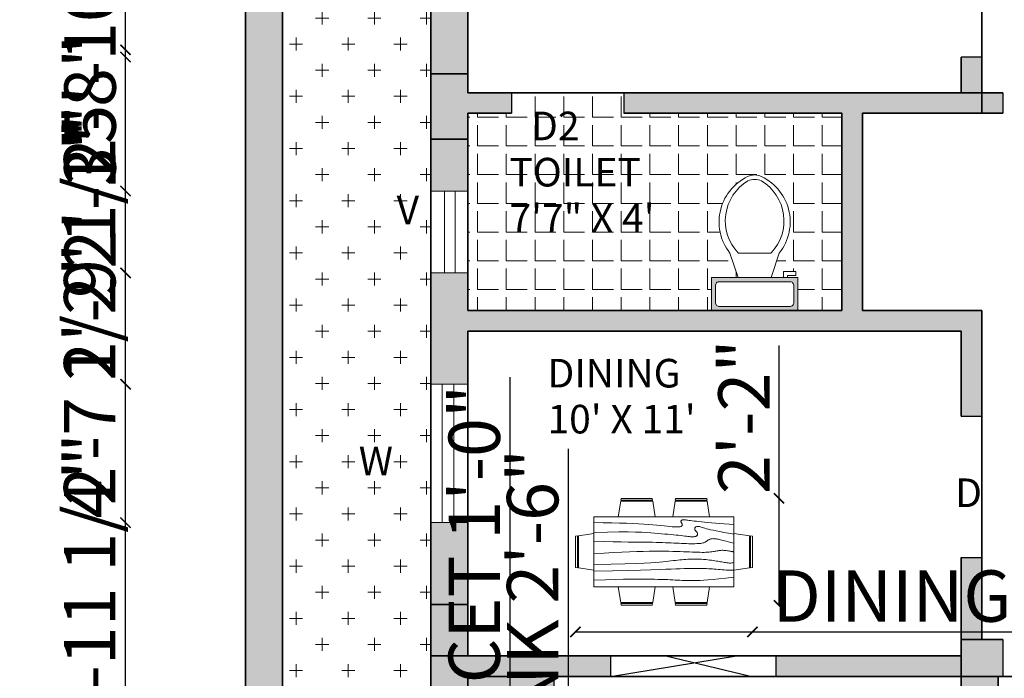
# Model space of a CAD drawing. Units: inches. Extents: x 1858 to 2399, y 1317 to 1943.
# Tile 2 of 8: x 1858 to 2098, y 1554 to 1714. Entities that reach past the tile are written whole.
import ezdxf

# ---------------------------------------------------------------- set-up
doc = ezdxf.new("R2010")
doc.units = ezdxf.units.IN
for name, color, linetype, lineweight in [('A-ANNO-DIMS', 2, 'Continuous', 18), ('A-ANNO-TEXT', 7, 'Continuous', 18), ('A-AREA-IDEN', 7, 'Continuous', 18), ('A-COLS', 7, 'Continuous', 35), ('A-COLS-PATT', 5, 'Continuous', 13), ('A-DOOR', 4, 'Continuous', 25), ('A-FLOR-CASE', 8, 'Continuous', 25), ('A-FLOR-FIXT', 9, 'Continuous', 18), ('A-FLOR-FIXT-PATT', 9, 'Continuous', 13), ('A-FLOR-PATT', 8, 'Continuous', 13), ('A-FURN', 8, 'Continuous', 18), ('A-WALL', 7, 'Continuous', 35), ('A-WALL-PATT', 1, 'Continuous', 13), ('L-SITE-PATT', 8, 'Continuous', 13), ('window', 4, 'Continuous', 18)]:
    doc.layers.add(name, color=color, linetype=linetype, lineweight=lineweight)
doc.styles.get("Standard").update_dxf_attribs({"font": 'arial.ttf'})
doc.dimstyles.new('ISO-25', dxfattribs={"dimtxt": 12.5, "dimasz": 2.5, "dimexe": 1.25, "dimexo": 0.625, "dimtad": 1, "dimdec": 0, "dimlunit": 4, "dimtxsty": 'Standard', "dimblk": 'ARCHTICK', "dimcen": 2.5, "dimse1": 1, "dimse2": 1, "dimclrd": 3, "dimclrt": 4, "dimadec": 0, "dimazin": 0, "dimtfac": 1, "dimtdec": 0, "dimtmove": 0, "dimatfit": 3, "dimfxl": 1, "dimarcsym": 0})

# ---------------------------------------------------------------- blocks, each defined once
blk = doc.blocks.new('*U4')
for p, q in [((9.5, -6), (9.5, -2)), ((-10, -8.5), (-8, -8.5)), ((-10, -9.5), (-10, -8.5)), ((-7, -9.5), (-10, -9.5)), ((-8, -8.5), (-8, -8)), ((-7, -8), (-7, -9.5)), ((-4, -8), (-6, -14)), ((4, -8), (6, -14)), ((4, -14), (-4, -14))]:
    blk.add_line(p, q)
blk.add_lwpolyline([(10.5, -8), (10.5, 0), (-10.5, 0), (-10.5, -8)], close=True)
for points in [[(-9.5, -2), (-9.5, -6)], [(8.5, -1), (-8.5, -1)], [(-8.5, -7), (8.5, -7)]]:
    blk.add_lwpolyline(points)
for centre, radius, start, end in [((-8.62, -1.88), 0.884, 81.8699, 188.1301), ((8.62, -1.88), 0.884, 351.8699, 98.1301), ((-8.62, -6.12), 0.884, 171.8699, 278.1301), ((8.62, -6.12), 0.884, 261.8699, 8.1301), ((3.52, -21.58), 12.17, 141.4691, 247.9714), ((4.2, -21.82), 11.33, 136.3677, 238.9468), ((-3.52, -21.58), 12.17, 292.0284, 38.5307), ((-4.2, -21.82), 11.33, 301.053, 43.6321), ((0, -27.88), 4, 245.7318, 294.2682), ((0, -29), 4, 254.8605, 285.1395)]:
    blk.add_arc(centre, radius, start, end)
blk = doc.blocks.new('Dining Set - 36 x 72 in.')
for p, q in [((-22.2343, 26.00059), (-23.4847, 17.99762)), ((-22.2304, 26), (-5.7608, 26)), ((-22, 27.5), (-22.1562, 26.50042)), ((-5.8416, 26.5), (-22.1534, 26.5)), ((-22, 27.5), (-6, 27.5)), ((-5.8437, 26.49966), (-6, 27.5)), ((-4.5152, 17.99762), (-5.7655, 25.99926)), ((5.7657, 26.00059), (4.5153, 17.99762)), ((5.7696, 26), (22.2392, 26)), ((6, 27.5), (5.8438, 26.50042)), ((22.1584, 26.5), (5.8466, 26.5)), ((6, 27.5), (22, 27.5)), ((22.1563, 26.49966), (22, 27.5)), ((23.4848, 17.99762), (22.2345, 25.99926)), ((36, 18), (-36, 18)), ((-36, 18), (-36, -18)), ((36, -18), (36, 18)), ((-45.5, 8), (-44.5004, 8.15617)), ((-45.5, 8), (-45.5, -8)), ((-44.5, -8.15843), (-44.5, 8.15338)), ((-44.0006, 8.23428), (-35.9976, 9.48474)), ((-44, 8.23041), (-44, -8.23915)), ((44.0006, 8.23428), (35.9976, 9.48474)), ((44, 8.23041), (44, -8.23915)), ((44.5, -8.15843), (44.5, 8.15338)), ((45.5, 8), (44.5005, 8.15617)), ((45.5, 8), (45.5, -8)), ((-44.4997, -8.15631), (-45.5, -8)), ((-35.9976, -9.48476), (-43.9993, -8.2345)), ((35.9976, -9.48476), (43.9993, -8.2345)), ((44.4997, -8.15631), (45.5, -8)), ((-36, -18), (36, -18)), ((-22.2343, -26.0006), (-23.4847, -17.99762)), ((-4.5152, -17.99762), (-5.7655, -25.99928)), ((5.7657, -26.0006), (4.5153, -17.99762)), ((23.4848, -17.99762), (22.2345, -25.99928)), ((-22.2304, -26), (-5.7608, -26)), ((-22, -27.5), (-22.1562, -26.50044)), ((-5.8416, -26.5), (-22.1534, -26.5)), ((-22, -27.5), (-6, -27.5)), ((-5.8437, -26.49967), (-6, -27.5)), ((5.7696, -26), (22.2392, -26)), ((6, -27.5), (5.8438, -26.50044)), ((22.1584, -26.5), (5.8466, -26.5)), ((6, -27.5), (22, -27.5)), ((22.1563, -26.49967), (22, -27.5))]:
    blk.add_line(p, q)
for points in [[(-36, 15), (-31.1772, 14.97754), (-26.8079, 14.91406), (-22.8538, 14.81543), (-19.276, 14.6875), (-16.0362, 14.53613), (-13.0957, 14.36718), (-10.4159, 14.18652), (-7.9583, 14), (-5.6904, 13.81315), (-3.6035, 13.63021), (-1.6954, 13.45508), (0.0365, 13.29166), (1.5945, 13.14388), (2.9811, 13.01562), (4.1988, 12.9108), (5.25, 12.83333), (6.1393, 12.78613), (6.8802, 12.76823), (7.4883, 12.77767), (7.9792, 12.8125), (8.3685, 12.87077), (8.6719, 12.95052), (8.9049, 13.0498), (9.0833, 13.16666), (9.2205, 13.29899), (9.3216, 13.44401), (9.3895, 13.59879), (9.4271, 13.76041), (9.4373, 13.92594), (9.4232, 14.09245), (9.3875, 14.257), (9.3333, 14.41666), (9.2638, 14.56917), (9.1836, 14.71484), (9.0975, 14.85465), (9.0104, 14.98958), (8.9272, 15.1206), (8.8529, 15.2487), (8.7922, 15.37483), (8.75, 15.5), (8.7305, 15.62467), (8.7344, 15.74739), (8.7617, 15.86621), (8.8125, 15.97916), (8.8867, 16.08431), (8.9844, 16.17968), (9.1055, 16.26334), (9.25, 16.33333), (9.4189, 16.38802), (9.6172, 16.42708), (9.8506, 16.45052), (10.125, 16.45833), (10.4463, 16.45052), (10.8203, 16.42708), (11.2529, 16.38802), (11.75, 16.33333), (12.3184, 16.26318), (12.9694, 16.17838), (13.7151, 16.07991), (14.5677, 15.96875), (15.5395, 15.84586), (16.6426, 15.71224), (17.8893, 15.56884), (19.2917, 15.41666), (20.859, 15.25667), (22.5879, 15.08984), (24.4721, 14.91715), (26.5052, 14.73958), (28.6809, 14.5581), (30.9929, 14.3737), (33.4347, 14.18733), (36, 14)], [(-36, 10), (-28.9766, 10.14274), (-23.1725, 10.20442), (-18.4241, 10.19775), (-14.5677, 10.13541), (-11.4399, 10.03011), (-8.877, 9.89453), (-6.7154, 9.74137), (-4.7917, 9.58333), (-2.9698, 9.43082), (-1.2246, 9.28515), (0.4415, 9.14534), (2.026, 9.01041), (3.5266, 8.87939), (4.9408, 8.7513), (6.266, 8.62516), (7.5, 8.5), (8.6411, 8.37549), (9.6914, 8.2539), (10.6538, 8.13818), (11.5312, 8.03125), (12.3267, 7.93603), (13.043, 7.85547), (13.6831, 7.79248), (14.25, 7.75), (14.7471, 7.7303), (15.1797, 7.73307), (15.5537, 7.75732), (15.875, 7.80208), (16.1494, 7.86637), (16.3828, 7.94922), (16.5811, 8.04964), (16.75, 8.16666), (16.8944, 8.29915), (17.0143, 8.44531), (17.1089, 8.60319), (17.1771, 8.77083), (17.218, 8.94629), (17.2305, 9.1276), (17.2137, 9.31282), (17.1667, 9.5), (17.0895, 9.6875), (16.987, 9.875), (16.8649, 10.0625), (16.7292, 10.25), (16.5856, 10.4375), (16.4401, 10.625), (16.2985, 10.8125), (16.1667, 11), (16.05, 11.18733), (15.9518, 11.3737), (15.8752, 11.5581), (15.8229, 11.73958), (15.798, 11.91715), (15.8034, 12.08984), (15.842, 12.25667), (15.9167, 12.41666), (16.0295, 12.56836), (16.1784, 12.70833), (16.3605, 12.83268), (16.5729, 12.9375), (16.8127, 13.01888), (17.0768, 13.07291), (17.3625, 13.0957), (17.6667, 13.08333), (17.9894, 13.03312), (18.3418, 12.94726), (18.7382, 12.82918), (19.1927, 12.68229), (19.7195, 12.51001), (20.3327, 12.31575), (21.0465, 12.10294), (21.875, 11.875), (22.8357, 11.63354), (23.959, 11.37304), (25.2786, 11.08618), (26.8282, 10.76562), (28.6414, 10.40405), (30.752, 9.99414), (33.1936, 9.52856), (36, 9)], [(-36, 5.5), (-30.7157, 5.3348), (-26.069, 5.20963), (-21.9946, 5.11767), (-18.4271, 5.05208), (-15.3009, 5.00602), (-12.5508, 4.97265), (-10.1112, 4.94515), (-7.9167, 4.91666), (-5.909, 4.88167), (-4.0586, 4.83984), (-2.3429, 4.79215), (-0.7396, 4.73958), (0.7739, 4.6831), (2.22, 4.6237), (3.6213, 4.56233), (5, 4.5), (6.373, 4.43782), (7.7344, 4.3776), (9.0723, 4.32129), (10.375, 4.27083), (11.6309, 4.22819), (12.8281, 4.19531), (13.9551, 4.17415), (15, 4.16666), (15.954, 4.17448), (16.819, 4.19791), (17.6001, 4.23698), (18.3021, 4.29166), (18.9299, 4.36198), (19.4883, 4.44791), (19.9823, 4.54948), (20.4167, 4.66666), (20.7969, 4.79899), (21.1302, 4.94401), (21.4245, 5.09879), (21.6875, 5.26041), (21.9271, 5.42594), (22.1511, 5.59245), (22.3672, 5.757), (22.5834, 5.91666), (22.8065, 6.06868), (23.0404, 6.21093), (23.2879, 6.34147), (23.5521, 6.45833), (23.8358, 6.55957), (24.142, 6.64323), (24.4735, 6.70735), (24.8334, 6.75), (25.2235, 6.76969), (25.642, 6.76692), (26.0858, 6.74267), (26.5521, 6.69791), (27.0379, 6.63362), (27.5404, 6.55078), (28.0565, 6.45036), (28.5834, 6.33333), (29.1242, 6.19987), (29.7071, 6.04687), (30.3661, 5.87044), (31.1354, 5.66666), (32.0493, 5.43164), (33.142, 5.16146), (34.4475, 4.85221), (36, 4.5)], [(-36, -1), (-30.7915, -0.6591), (-26.0195, -0.38216), (-21.6519, -0.16284), (-17.6563, 0.00521), (-14.0005, 0.12833), (-10.6523, 0.21289), (-7.5796, 0.26522), (-4.75, 0.29166), (-2.134, 0.29793), (0.2878, 0.28711), (2.5317, 0.26163), (4.6146, 0.22396), (6.5529, 0.17651), (8.3633, 0.12174), (10.0623, 0.06209), (11.6667, 0), (13.1899, -0.06201), (14.6341, -0.1211), (15.9982, -0.17432), (17.2813, -0.21875), (18.4823, -0.25147), (19.6003, -0.26953), (20.6343, -0.27002), (21.5834, -0.25), (22.4481, -0.20768), (23.2357, -0.14584), (23.9549, -0.06836), (24.6146, 0.02083), (25.2235, 0.11784), (25.7904, 0.21875), (26.3241, 0.31966), (26.8334, 0.41666), (27.3265, 0.50618), (27.8099, 0.58593), (28.2894, 0.65397), (28.7709, 0.70833), (29.2601, 0.74707), (29.763, 0.76823), (30.2855, 0.76985), (30.8334, 0.75), (31.4088, 0.70784), (31.9994, 0.64713), (32.589, 0.57275), (33.1615, 0.48958), (33.7008, 0.4025), (34.1908, 0.3164), (34.6153, 0.23616), (34.9584, 0.16666), (35.2099, 0.11165), (35.3848, 0.07031), (35.504, 0.04069), (35.5886, 0.02083), (35.6594, 0.00879), (35.7377, 0.0026), (35.8442, 0.00032), (36, 0)], [(-36, -6.5), (-27.1843, -6.31267), (-20.084, -6.1263), (-14.469, -5.9419), (-10.1094, -5.76042), (-6.7752, -5.58285), (-4.2363, -5.41016), (-2.2629, -5.24333), (-0.625, -5.08334), (0.8708, -4.93099), (2.2715, -4.78646), (3.5872, -4.64974), (4.8281, -4.52084), (6.0046, -4.39974), (7.127, -4.28646), (8.2053, -4.18099), (9.25, -4.08334), (10.2705, -3.99382), (11.2734, -3.91407), (12.2647, -3.84603), (13.25, -3.79167), (14.2354, -3.75293), (15.2266, -3.73177), (16.2295, -3.73015), (17.25, -3.75), (18.2912, -3.79248), (19.3451, -3.85547), (20.4009, -3.93604), (21.4479, -4.03125), (22.4754, -4.13819), (23.4727, -4.25391), (24.4289, -4.37549), (25.3334, -4.5), (26.1785, -4.62492), (26.9694, -4.74935), (27.7145, -4.87281), (28.4219, -4.99479), (29.1, -5.11483), (29.7572, -5.23242), (30.4016, -5.34709), (31.0417, -5.45834), (31.6837, -5.56437), (32.3262, -5.65821), (32.9658, -5.73153), (33.599, -5.77604), (34.2224, -5.78345), (34.8327, -5.74545), (35.4264, -5.65373), (36, -5.5)], [(-36, -10), (-26.4022, -9.81299), (-18.4675, -9.62891), (-11.9839, -9.45069), (-6.7396, -9.28125), (-2.5226, -9.12354), (0.8789, -8.98047), (3.6769, -8.85498), (6.0833, -8.75), (8.2767, -8.66765), (10.3021, -8.60677), (12.1712, -8.56543), (13.8958, -8.54167), (15.4876, -8.53353), (16.9583, -8.53907), (18.3197, -8.55632), (19.5834, -8.58334), (20.7616, -8.61841), (21.8685, -8.66081), (22.9188, -8.71004), (23.9271, -8.76563), (24.9081, -8.82707), (25.8763, -8.89388), (26.8465, -8.96558), (27.8334, -9.04167), (28.8474, -9.12118), (29.8828, -9.20117), (30.93, -9.27824), (31.9792, -9.34896), (33.0205, -9.40991), (34.0443, -9.45768), (35.0407, -9.48885), (36, -9.5)], [(-36, -14.5), (-30.0881, -14.33513), (-25.0332, -14.21224), (-20.7312, -14.12647), (-17.0781, -14.07292), (-13.97, -14.04671), (-11.3027, -14.04297), (-8.9724, -14.05681), (-6.875, -14.08334), (-4.9224, -14.11833), (-3.0905, -14.16016), (-1.3709, -14.20785), (0.2448, -14.26042), (1.7647, -14.3169), (3.1973, -14.3763), (4.5507, -14.43767), (5.8333, -14.5), (7.0554, -14.5621), (8.235, -14.62175), (9.3922, -14.67652), (10.5469, -14.72396), (11.7192, -14.76164), (12.929, -14.78711), (14.1965, -14.79794), (15.5417, -14.79167), (16.9933, -14.76424), (18.6152, -14.70508), (20.4804, -14.60197), (22.6615, -14.44271), (25.2312, -14.21509), (28.2624, -13.9069), (31.8277, -13.50594), (36, -13)]]:
    blk.add_lwpolyline(points)
blk = doc.blocks.new('_ArchTick')
at = {"color": 0, "linetype": 'ByBlock', "const_width": 0.15}
blk.add_lwpolyline([(-0.5, -0.5), (0.5, 0.5)], dxfattribs=at)
blk = doc.blocks.new('*D21')
at = {"layer": 'A-ANNO-DIMS', "color": 3, "lineweight": -2, "transparency": 16777216}
for p, q in [((1991.88, 1527.2), (1991.88, 1609.72)), ((1991.88, 1497.2), (1991.88, 1527.2))]:
    blk.add_line(p, q, dxfattribs=at)
at = {"layer": 'Defpoints', "color": 0, "transparency": 16777216}
for p in [(1987.38, 1527.2), (1991.88, 1527.2), (1987.38, 1497.2)]:
    blk.add_point(p, dxfattribs=at)
at = {"layer": 'A-ANNO-DIMS', "color": 3, "lineweight": -2, "transparency": 16777216, "xscale": 2.5, "yscale": 2.5, "zscale": 2.5}
for p, rotation in [((1991.88, 1527.2), 90), ((1991.88, 1497.2), 270)]:
    blk.add_blockref('_ArchTick', p, dxfattribs=dict(at, rotation=rotation))
at = {"layer": 'A-ANNO-DIMS', "color": 4, "transparency": 16777216, "insert": (1984.79, 1569.71), "char_height": 12.5, "attachment_point": 5, "rotation": 90}
blk.add_mtext('SINK 2\'-6"', dxfattribs=at)
blk = doc.blocks.new('*D23')
at = {"layer": 'A-ANNO-DIMS', "color": 3, "lineweight": -2, "transparency": 16777216}
for p, q in [((1977.68, 1516.18), (1977.68, 1627.15)), ((1977.68, 1504.18), (1977.68, 1516.18))]:
    blk.add_line(p, q, dxfattribs=at)
at = {"layer": 'Defpoints', "color": 0, "transparency": 16777216}
for p in [(1975.88, 1516.18), (1977.68, 1516.18), (1975.88, 1504.18)]:
    blk.add_point(p, dxfattribs=at)
at = {"layer": 'A-ANNO-DIMS', "color": 3, "lineweight": -2, "transparency": 16777216, "xscale": 2.5, "yscale": 2.5, "zscale": 2.5}
for p, rotation in [((1977.68, 1516.18), 90), ((1977.68, 1504.18), 270)]:
    blk.add_blockref('_ArchTick', p, dxfattribs=dict(at, rotation=rotation))
at = {"layer": 'A-ANNO-DIMS', "color": 4, "transparency": 16777216, "insert": (1970.59, 1572.91), "char_height": 12.5, "attachment_point": 5, "rotation": 90}
blk.add_mtext('FAUCET 1\'-0"', dxfattribs=at)
blk = doc.blocks.new('*D25')
at = {"layer": 'A-ANNO-DIMS', "color": 3, "lineweight": -2, "transparency": 16777216}
for p, q in [((1993.57, 1565.17), (2036.62, 1565.17)), ((2036.62, 1565.17), (2177.76, 1565.17))]:
    blk.add_line(p, q, dxfattribs=at)
at = {"layer": 'Defpoints', "color": 0, "transparency": 16777216}
for p in [(1993.57, 1571.63), (2036.62, 1571.63), (2036.62, 1565.17)]:
    blk.add_point(p, dxfattribs=at)
at = {"layer": 'A-ANNO-DIMS', "color": 3, "lineweight": -2, "transparency": 16777216, "xscale": 2.5, "yscale": 2.5, "zscale": 2.5, "rotation": 180}
blk.add_blockref('_ArchTick', (1993.57, 1565.17), dxfattribs=at)
at = {"layer": 'A-ANNO-DIMS', "color": 3, "lineweight": -2, "transparency": 16777216, "xscale": 2.5, "yscale": 2.5, "zscale": 2.5}
blk.add_blockref('_ArchTick', (2036.62, 1565.17), dxfattribs=at)
at = {"layer": 'A-ANNO-DIMS', "color": 4, "transparency": 16777216, "insert": (2108.44, 1572.26), "char_height": 12.5, "attachment_point": 5}
blk.add_mtext('DINING SET 3\'-7"', dxfattribs=at)
blk = doc.blocks.new('*D26')
at = {"layer": 'A-ANNO-DIMS', "color": 3, "lineweight": -2, "transparency": 16777216}
for p, q in [((2043.08, 1597.65), (2043.08, 1634.84)), ((2043.08, 1571.63), (2043.08, 1597.65))]:
    blk.add_line(p, q, dxfattribs=at)
at = {"layer": 'Defpoints', "color": 0, "transparency": 16777216}
for p in [(2036.62, 1597.65), (2043.08, 1597.65), (2036.62, 1571.63)]:
    blk.add_point(p, dxfattribs=at)
at = {"layer": 'A-ANNO-DIMS', "color": 3, "lineweight": -2, "transparency": 16777216, "xscale": 2.5, "yscale": 2.5, "zscale": 2.5}
for p, rotation in [((2043.08, 1597.65), 90), ((2043.08, 1571.63), 270)]:
    blk.add_blockref('_ArchTick', p, dxfattribs=dict(at, rotation=rotation))
at = {"layer": 'A-ANNO-DIMS', "color": 4, "transparency": 16777216, "insert": (2036.18, 1617.49), "char_height": 12.5, "attachment_point": 5, "rotation": 90}
blk.add_mtext('2\'-2"', dxfattribs=at)
blk = doc.blocks.new('*D31')
at = {"layer": 'A-ANNO-DIMS', "color": 3, "lineweight": -2, "transparency": 16777216}
for p, q in [((1967.38, 1917.54), (1988.35, 1917.54)), ((1988.35, 1917.54), (2024.15, 1917.54))]:
    blk.add_line(p, q, dxfattribs=at)
at = {"layer": 'Defpoints', "color": 0, "transparency": 16777216}
for p in [(1988.35, 1917.54), (1967.38, 1554.34), (1988.35, 1554.34)]:
    blk.add_point(p, dxfattribs=at)
at = {"layer": 'A-ANNO-DIMS', "color": 3, "lineweight": -2, "transparency": 16777216, "xscale": 2.5, "yscale": 2.5, "zscale": 2.5, "rotation": 180}
blk.add_blockref('_ArchTick', (1967.38, 1917.54), dxfattribs=at)
at = {"layer": 'A-ANNO-DIMS', "color": 3, "lineweight": -2, "transparency": 16777216, "xscale": 2.5, "yscale": 2.5, "zscale": 2.5}
blk.add_blockref('_ArchTick', (1988.35, 1917.54), dxfattribs=at)
at = {"layer": 'A-ANNO-DIMS', "color": 4, "transparency": 16777216, "insert": (2007.5, 1924.55), "char_height": 12.5, "attachment_point": 5}
blk.add_mtext('1\'-9"', dxfattribs=at)
blk = doc.blocks.new('*D40')
at = {"layer": 'A-ANNO-DIMS', "color": 3, "lineweight": -2, "transparency": 16777216}
for p, q in [((1884.18, 1536.07), (1884.18, 1611.87)), ((1884.18, 1488.33), (1884.18, 1536.07))]:
    blk.add_line(p, q, dxfattribs=at)
at = {"layer": 'Defpoints', "color": 0, "transparency": 16777216}
for p in [(1884.18, 1536.07), (1958.38, 1536.07), (1958.38, 1488.33)]:
    blk.add_point(p, dxfattribs=at)
at = {"layer": 'A-ANNO-DIMS', "color": 3, "lineweight": -2, "transparency": 16777216, "xscale": 2.5, "yscale": 2.5, "zscale": 2.5}
for p, rotation in [((1884.18, 1536.07), 90), ((1884.18, 1488.33), 270)]:
    blk.add_blockref('_ArchTick', p, dxfattribs=dict(at, rotation=rotation))
at = {"layer": 'A-ANNO-DIMS', "color": 4, "transparency": 16777216, "insert": (1877.08, 1575.22), "char_height": 12.5, "attachment_point": 5, "rotation": 90}
blk.add_mtext('3\'-11 1/2"', dxfattribs=at)
blk = doc.blocks.new('*D41')
at = {"layer": 'A-ANNO-DIMS', "color": 3, "lineweight": -2, "transparency": 16777216}
for p, q in [((1884.18, 1591.74), (1884.18, 1658.34)), ((1884.18, 1536.07), (1884.18, 1591.74))]:
    blk.add_line(p, q, dxfattribs=at)
at = {"layer": 'Defpoints', "color": 0, "transparency": 16777216}
for p in [(1884.18, 1591.74), (1958.38, 1591.74), (1958.38, 1536.07)]:
    blk.add_point(p, dxfattribs=at)
at = {"layer": 'A-ANNO-DIMS', "color": 3, "lineweight": -2, "transparency": 16777216, "xscale": 2.5, "yscale": 2.5, "zscale": 2.5}
for p, rotation in [((1884.18, 1591.74), 90), ((1884.18, 1536.07), 270)]:
    blk.add_blockref('_ArchTick', p, dxfattribs=dict(at, rotation=rotation))
at = {"layer": 'A-ANNO-DIMS', "color": 4, "transparency": 16777216, "insert": (1877.09, 1626.29), "char_height": 12.5, "attachment_point": 5, "rotation": 90}
blk.add_mtext('4\'-7 1/2"', dxfattribs=at)
blk = doc.blocks.new('*D42')
at = {"layer": 'A-ANNO-DIMS', "color": 3, "lineweight": -2, "transparency": 16777216}
for p, q in [((1884.18, 1625.4), (1884.18, 1691.71)), ((1884.18, 1591.74), (1884.18, 1625.4))]:
    blk.add_line(p, q, dxfattribs=at)
at = {"layer": 'Defpoints', "color": 0, "transparency": 16777216}
for p in [(1884.18, 1625.4), (1958.38, 1625.4), (1958.38, 1591.74)]:
    blk.add_point(p, dxfattribs=at)
at = {"layer": 'A-ANNO-DIMS', "color": 3, "lineweight": -2, "transparency": 16777216, "xscale": 2.5, "yscale": 2.5, "zscale": 2.5}
for p, rotation in [((1884.18, 1625.4), 90), ((1884.18, 1591.74), 270)]:
    blk.add_blockref('_ArchTick', p, dxfattribs=dict(at, rotation=rotation))
at = {"layer": 'A-ANNO-DIMS', "color": 4, "transparency": 16777216, "insert": (1877.09, 1659.8), "char_height": 12.5, "attachment_point": 5, "rotation": 90}
blk.add_mtext('2\'-9 1/2"', dxfattribs=at)
blk = doc.blocks.new('*D43')
at = {"layer": 'A-ANNO-DIMS', "color": 3, "lineweight": -2, "transparency": 16777216}
for p, q in [((1884.18, 1652.51), (1884.18, 1689.7)), ((1884.18, 1625.4), (1884.18, 1652.51))]:
    blk.add_line(p, q, dxfattribs=at)
at = {"layer": 'Defpoints', "color": 0, "transparency": 16777216}
for p in [(1884.18, 1652.51), (1958.38, 1652.51), (1958.38, 1625.4)]:
    blk.add_point(p, dxfattribs=at)
at = {"layer": 'A-ANNO-DIMS', "color": 3, "lineweight": -2, "transparency": 16777216, "xscale": 2.5, "yscale": 2.5, "zscale": 2.5}
for p, rotation in [((1884.18, 1652.51), 90), ((1884.18, 1625.4), 270)]:
    blk.add_blockref('_ArchTick', p, dxfattribs=dict(at, rotation=rotation))
at = {"layer": 'A-ANNO-DIMS', "color": 4, "transparency": 16777216, "insert": (1877.16, 1672.36), "char_height": 12.5, "attachment_point": 5, "rotation": 90}
blk.add_mtext('2\'-3"', dxfattribs=at)
blk = doc.blocks.new('*D44')
at = {"layer": 'A-ANNO-DIMS', "color": 3, "lineweight": -2, "transparency": 16777216}
for p, q in [((1884.18, 1672.42), (1884.18, 1708.22)), ((1884.18, 1652.51), (1884.18, 1672.42))]:
    blk.add_line(p, q, dxfattribs=at)
at = {"layer": 'Defpoints', "color": 0, "transparency": 16777216}
for p in [(1884.18, 1672.42), (1958.38, 1672.42), (1958.38, 1652.51)]:
    blk.add_point(p, dxfattribs=at)
at = {"layer": 'A-ANNO-DIMS', "color": 3, "lineweight": -2, "transparency": 16777216, "xscale": 2.5, "yscale": 2.5, "zscale": 2.5}
for p, rotation in [((1884.18, 1672.42), 90), ((1884.18, 1652.51), 270)]:
    blk.add_blockref('_ArchTick', p, dxfattribs=dict(at, rotation=rotation))
at = {"layer": 'A-ANNO-DIMS', "color": 4, "transparency": 16777216, "insert": (1877.17, 1691.57), "char_height": 12.5, "attachment_point": 5, "rotation": 90}
blk.add_mtext('1\'-8"', dxfattribs=at)
blk = doc.blocks.new('*D45')
at = {"layer": 'A-ANNO-DIMS', "color": 3, "lineweight": -2, "transparency": 16777216}
blk.add_line((1884.18, 1672.42), (1884.18, 1742.58), dxfattribs=at)
at = {"layer": 'Defpoints', "color": 0, "transparency": 16777216}
for p in [(1884.18, 1742.58), (1958.38, 1742.58), (1958.38, 1672.42)]:
    blk.add_point(p, dxfattribs=at)
at = {"layer": 'A-ANNO-DIMS', "color": 3, "lineweight": -2, "transparency": 16777216, "xscale": 2.5, "yscale": 2.5, "zscale": 2.5}
for p, rotation in [((1884.18, 1742.58), 90), ((1884.18, 1672.42), 270)]:
    blk.add_blockref('_ArchTick', p, dxfattribs=dict(at, rotation=rotation))
at = {"layer": 'A-ANNO-DIMS', "color": 4, "transparency": 16777216, "insert": (1877.17, 1707.5), "char_height": 12.5, "attachment_point": 5, "rotation": 90}
blk.add_mtext('5\'-10"', dxfattribs=at)
blk = doc.blocks.new('*D50')
at = {"layer": 'A-ANNO-DIMS', "color": 3, "lineweight": -2, "transparency": 16777216}
for p, q in [((2097.46, 1917.54), (2127.41, 1917.54)), ((2127.41, 1917.54), (2164.6, 1917.54))]:
    blk.add_line(p, q, dxfattribs=at)
at = {"layer": 'Defpoints', "color": 0, "transparency": 16777216}
for p in [(2127.41, 1917.54), (2097.46, 1563.34), (2127.41, 1563.34)]:
    blk.add_point(p, dxfattribs=at)
at = {"layer": 'A-ANNO-DIMS', "color": 3, "lineweight": -2, "transparency": 16777216, "xscale": 2.5, "yscale": 2.5, "zscale": 2.5, "rotation": 180}
blk.add_blockref('_ArchTick', (2097.46, 1917.54), dxfattribs=at)
at = {"layer": 'A-ANNO-DIMS', "color": 3, "lineweight": -2, "transparency": 16777216, "xscale": 2.5, "yscale": 2.5, "zscale": 2.5}
blk.add_blockref('_ArchTick', (2127.41, 1917.54), dxfattribs=at)
at = {"layer": 'A-ANNO-DIMS', "color": 4, "transparency": 16777216, "insert": (2147.25, 1924.55), "char_height": 12.5, "attachment_point": 5}
blk.add_mtext('2\'-6"', dxfattribs=at)
blk = doc.blocks.new('*D56')
at = {"layer": 'A-ANNO-DIMS', "color": 3, "lineweight": -2, "transparency": 16777216}
for p, q in [((1977.99, 1917.54), (2005.38, 1917.54)), ((2005.38, 1917.54), (2071.7, 1917.54))]:
    blk.add_line(p, q, dxfattribs=at)
at = {"layer": 'Defpoints', "color": 0, "transparency": 16777216}
for p in [(2005.38, 1917.54), (1977.99, 1696.34), (2005.38, 1696.34)]:
    blk.add_point(p, dxfattribs=at)
at = {"layer": 'A-ANNO-DIMS', "color": 3, "lineweight": -2, "transparency": 16777216, "xscale": 2.5, "yscale": 2.5, "zscale": 2.5, "rotation": 180}
blk.add_blockref('_ArchTick', (1977.99, 1917.54), dxfattribs=at)
at = {"layer": 'A-ANNO-DIMS', "color": 3, "lineweight": -2, "transparency": 16777216, "xscale": 2.5, "yscale": 2.5, "zscale": 2.5}
blk.add_blockref('_ArchTick', (2005.38, 1917.54), dxfattribs=at)
at = {"layer": 'A-ANNO-DIMS', "color": 4, "transparency": 16777216, "insert": (2039.79, 1924.63), "char_height": 12.5, "attachment_point": 5}
blk.add_mtext('2\'-3 1/2"', dxfattribs=at)
blk = doc.blocks.new('*D57')
at = {"layer": 'A-ANNO-DIMS', "color": 3, "lineweight": -2, "transparency": 16777216}
for p, q in [((1884.18, 1729.93), (1884.18, 1767.12)), ((1884.18, 1705.02), (1884.18, 1729.93))]:
    blk.add_line(p, q, dxfattribs=at)
at = {"layer": 'Defpoints', "color": 0, "transparency": 16777216}
for p in [(1884.18, 1729.93), (2087.38, 1729.93), (2087.38, 1705.02)]:
    blk.add_point(p, dxfattribs=at)
at = {"layer": 'A-ANNO-DIMS', "color": 3, "lineweight": -2, "transparency": 16777216, "xscale": 2.5, "yscale": 2.5, "zscale": 2.5}
for p, rotation in [((1884.18, 1729.93), 90), ((1884.18, 1705.02), 270)]:
    blk.add_blockref('_ArchTick', p, dxfattribs=dict(at, rotation=rotation))
at = {"layer": 'A-ANNO-DIMS', "color": 4, "transparency": 16777216, "insert": (1877.28, 1749.77), "char_height": 12.5, "attachment_point": 5, "rotation": 90}
blk.add_mtext('2\'-1"', dxfattribs=at)
blk = doc.blocks.new('*D58')
at = {"layer": 'A-ANNO-DIMS', "color": 3, "lineweight": -2, "transparency": 16777216}
for p, q in [((1884.18, 1730.57), (1884.18, 1767.76)), ((1884.18, 1706.78), (1884.18, 1730.57))]:
    blk.add_line(p, q, dxfattribs=at)
at = {"layer": 'Defpoints', "color": 0, "transparency": 16777216}
for p in [(1884.18, 1730.57), (2145.38, 1730.57), (2145.38, 1706.78)]:
    blk.add_point(p, dxfattribs=at)
at = {"layer": 'A-ANNO-DIMS', "color": 3, "lineweight": -2, "transparency": 16777216, "xscale": 2.5, "yscale": 2.5, "zscale": 2.5}
for p, rotation in [((1884.18, 1730.57), 90), ((1884.18, 1706.78), 270)]:
    blk.add_blockref('_ArchTick', p, dxfattribs=dict(at, rotation=rotation))
at = {"layer": 'A-ANNO-DIMS', "color": 4, "transparency": 16777216, "insert": (1877.17, 1750.41), "char_height": 12.5, "attachment_point": 5, "rotation": 90}
blk.add_mtext('2\'-0"', dxfattribs=at)
blk = doc.blocks.new('*D59')
at = {"layer": 'A-ANNO-DIMS', "color": 3, "lineweight": -2, "transparency": 16777216}
for p, q in [((2302.58, 1617.63), (2302.58, 1693.66)), ((2302.58, 1583.24), (2302.58, 1617.63))]:
    blk.add_line(p, q, dxfattribs=at)
at = {"layer": 'Defpoints', "color": 0, "transparency": 16777216}
for p in [(2092.38, 1617.63), (2302.58, 1617.63), (2092.38, 1583.24)]:
    blk.add_point(p, dxfattribs=at)
at = {"layer": 'A-ANNO-DIMS', "color": 3, "lineweight": -2, "transparency": 16777216, "xscale": 2.5, "yscale": 2.5, "zscale": 2.5}
for p, rotation in [((2302.58, 1617.63), 90), ((2302.58, 1583.24), 270)]:
    blk.add_blockref('_ArchTick', p, dxfattribs=dict(at, rotation=rotation))
at = {"layer": 'A-ANNO-DIMS', "color": 4, "transparency": 16777216, "insert": (2295.49, 1656.89), "char_height": 12.5, "attachment_point": 5, "rotation": 90}
blk.add_mtext('2\'-10 1/2"', dxfattribs=at)

msp = doc.modelspace()

# ---------------------------------------------------------------- hatches: boundary and pattern name
at = {"layer": 'A-COLS-PATT'}
h = msp.add_hatch(color=256, dxfattribs=at)
h.dxf.hatch_style = 1
h.paths.add_polyline_path([(1977.99, 1696.34), (1967.38, 1696.34), (1967.38, 1700.89), (1958.38, 1700.89), (1958.38, 1685.05), (1967.38, 1685.05), (1967.38, 1691.34), (1977.99, 1691.34)])
h.paths.add_polyline_path([(1967.38, 1571.83), (1958.38, 1571.83), (1958.38, 1559.34), (1967.38, 1559.34)])
h.paths.add_polyline_path([(1977.97, 1476.34), (1967.38, 1476.34), (1967.38, 1482.01), (1958.38, 1474.25), (1958.38, 1467.34), (1967.38, 1467.34)])
h.paths.add_polyline_path([(2096.38, 1473.96), (2087.38, 1481.51), (2087.38, 1476.34), (2084.48, 1476.34), (2089.85, 1467.34), (2096.38, 1467.34)])
h.paths.add_polyline_path([(2273.38, 1837.34), (2265.79, 1837.34), (2258.24, 1828.34), (2264.38, 1828.34), (2264.38, 1823.36), (2273.38, 1827.14)])
h.paths.add_polyline_path([(2097.64, 1837.34), (2082.58, 1837.34), (2082.58, 1828.34), (2097.64, 1828.34)])
h.paths.add_polyline_path([(1977.66, 1837.34), (1949.42, 1837.34), (1949.42, 1828.34), (1977.66, 1828.34)])
h = msp.add_hatch(color=256, dxfattribs=at)
h.dxf.hatch_style = 1
h.paths.add_polyline_path([(2092.38, 1705.02), (2087.38, 1705.02), (2087.38, 1696.34), (2092.38, 1696.34)])
h.paths.add_polyline_path([(2097.51, 1696.34), (2092.38, 1696.34), (2092.38, 1691.34), (2097.51, 1691.34)])
h.paths.add_polyline_path([(2140.38, 1696.34), (2135.36, 1696.34), (2135.36, 1691.34), (2140.38, 1691.34)])
h.paths.add_polyline_path([(2145.38, 1706.78), (2140.38, 1706.78), (2140.38, 1696.34), (2145.38, 1696.34)])
h.paths.add_polyline_path([(2097.46, 1563.34), (2092.38, 1563.34), (2087.38, 1563.34), (2087.38, 1554.34), (2096.38, 1554.34), (2097.46, 1554.34)])
at = {"layer": 'A-FLOR-FIXT-PATT'}
h = msp.add_hatch(color=256, dxfattribs=at)
h.dxf.hatch_style = 1
h.set_gradient(color1=(0, 0, 255), color2=(255, 255, 0))
h.paths.add_polyline_path([(2010.03, 1501.34), (2040.03, 1501.34), (2040.03, 1477.34), (2034.03, 1477.34), (2034.03, 1476.34), (2038.03, 1476.34), (2050.44, 1476.34), (2056.5, 1476.34), (2056.5, 1507.28), (1988.35, 1507.28), (1988.35, 1554.34), (1967.38, 1554.34), (1967.38, 1525.7, -0.414214), (1968.88, 1527.2), (1985.88, 1527.2, -0.414214), (1987.38, 1525.7), (1987.38, 1498.7, -0.414214), (1985.88, 1497.2), (1968.88, 1497.2, -0.414214), (1967.38, 1498.7), (1967.38, 1476.34), (2016.03, 1476.34), (2016.03, 1477.34), (2010.03, 1477.34)])
h.paths.add_polyline_path([(2129, 1826.59, 0.414214), (2128, 1827.34), (2110.75, 1827.34, 0.414214), (2110, 1826.34), (2110, 1822.09, 0.414214), (2111, 1821.34), (2128.25, 1821.34, 0.414214), (2129, 1822.34)])
h.paths.add_polyline_path([(2047.65, 1651.34), (2026.65, 1651.34), (2026.65, 1643.34), (2047.65, 1643.34)])
h.paths.add_polyline_path([(2045.65, 1644.34, 0.5), (2046.65, 1645.34), (2046.65, 1649.34, 0.5), (2045.65, 1650.34), (2028.65, 1650.34, 0.5), (2027.65, 1649.34), (2027.65, 1645.34, 0.5), (2028.65, 1644.34)], flags=16)
at = {"layer": 'A-FLOR-PATT'}
h = msp.add_hatch(dxfattribs=at)
h.set_pattern_fill('ANGLE', color=256)
h.set_pattern_definition([(0, (0, 0), (0, 6.985), [5.08, -1.905]), (90, (0, 0), (-6.985, 4e-16), [5.08, -1.905])])
h.paths.add_polyline_path([(2058.38, 1691.34), (2005.38, 1691.34), (2005.38, 1696.34), (1977.99, 1696.34), (1977.99, 1691.34), (1967.38, 1691.34), (1967.38, 1643.34), (2026.65, 1643.34), (2026.65, 1651.34), (2033.15, 1651.34), (2031.15, 1657.34, -0.501323), (2036.1, 1676.2, -0.132891), (2038.19, 1676.2, -0.501317), (2043.15, 1657.34), (2041.15, 1651.34), (2044.15, 1651.34), (2044.15, 1652.84), (2047.15, 1652.84), (2047.15, 1651.34), (2047.65, 1651.34), (2047.65, 1643.34), (2058.38, 1643.34)])
h.paths.add_polyline_path([(2140.38, 1828.34), (2130, 1828.34), (2130, 1820.34), (2123.5, 1820.34), (2125.5, 1814.34, -0.501323), (2120.55, 1795.48, -0.132891), (2118.46, 1795.48, -0.501317), (2113.5, 1814.34), (2115.5, 1820.34), (2112.5, 1820.34), (2112.5, 1818.84), (2109.5, 1818.84), (2109.5, 1820.34), (2109, 1820.34), (2109, 1828.34), (2107.67, 1828.34), (2092.38, 1828.34), (2092.38, 1744.34), (2140.38, 1744.34)])
h.paths.add_polyline_path([(1981.03, 1683.02), (1996.96, 1683.02), (1996.96, 1693.5), (1981.03, 1693.5)], flags=24)
h.paths.add_polyline_path([(1975.79, 1660.59), (2014.55, 1660.59), (2014.55, 1671.04), (1975.79, 1671.04)], flags=24)
h.paths.add_polyline_path([(1975.73, 1671.6), (2013.37, 1671.6), (2013.37, 1682.41), (1975.73, 1682.41)], flags=24)
h.paths.add_polyline_path([(2096.15, 1778.17), (2126.05, 1778.17), (2126.05, 1788.61), (2096.15, 1788.61)], flags=24)
h.paths.add_polyline_path([(2096.09, 1789.17), (2133.73, 1789.17), (2133.73, 1799.98), (2096.09, 1799.98)], flags=24)
at = {"layer": 'A-WALL-PATT'}
h = msp.add_hatch(color=256, dxfattribs=at)
h.dxf.hatch_style = 1
h.paths.add_polyline_path([(1967.38, 1742.58), (1958.38, 1742.58), (1958.38, 1700.89), (1967.38, 1700.89)])
h.paths.add_polyline_path([(1967.38, 1685.05), (1958.38, 1685.05), (1958.38, 1672.42), (1967.38, 1672.42)], flags=17)
h.paths.add_polyline_path([(2092.38, 1643.34), (2087.38, 1643.34), (2063.38, 1643.34), (2063.38, 1691.34), (2087.38, 1691.34), (2092.38, 1691.34), (2092.38, 1696.34), (2087.38, 1696.34), (2005.38, 1696.34), (2005.38, 1691.34), (2058.38, 1691.34), (2058.38, 1643.34), (1967.38, 1643.34), (1967.38, 1652.51), (1958.38, 1652.51), (1958.38, 1625.4), (1967.38, 1625.4), (1967.38, 1638.34), (2087.38, 1638.34), (2087.38, 1617.63), (2092.38, 1617.63)])
h.paths.add_polyline_path([(1967.38, 1591.74), (1958.38, 1591.74), (1958.38, 1571.83), (1967.38, 1571.83)])
h.paths.add_polyline_path([(1967.38, 1554.34), (2002.1, 1554.34), (2002.1, 1559.34), (1967.38, 1559.34), (1958.38, 1559.34), (1958.38, 1536.07), (1967.38, 1536.07)])
h.paths.add_polyline_path([(2087.38, 1559.34), (2042.3, 1559.34), (2042.3, 1554.34), (2087.38, 1554.34)])
h.paths.add_polyline_path([(2092.38, 1583.24), (2087.38, 1583.24), (2087.38, 1563.34), (2092.38, 1563.34)])
h.paths.add_polyline_path([(2096.38, 1554.34), (2087.38, 1554.34), (2087.38, 1481.51), (2096.38, 1473.96)])
h.paths.add_polyline_path([(2084.48, 1476.34), (2050.44, 1476.34), (2050.44, 1467.34), (2089.85, 1467.34)])
h.paths.add_polyline_path([(2002.33, 1476.34), (1977.97, 1476.34), (1967.38, 1467.34), (2002.33, 1467.34)])
h.paths.add_polyline_path([(1967.38, 1488.33), (1958.38, 1488.33), (1958.38, 1474.25), (1967.38, 1482.01)])
h.paths.add_polyline_path([(2121.99, 1554.34), (2119.71, 1554.34), (2119.71, 1532.61), (2096.38, 1532.61), (2096.38, 1529.65), (2121.99, 1529.65)])
h.paths.add_polyline_path([(2171.86, 1563.34), (2127.41, 1563.34), (2127.41, 1554.34), (2171.86, 1554.34)])
h.paths.add_polyline_path([(2264.38, 1563.34), (2220, 1563.34), (2220, 1554.34), (2264.38, 1554.34)])
h.paths.add_polyline_path([(2273.38, 1563.34), (2264.38, 1563.34), (2264.38, 1366.34), (2241.64, 1366.34), (2241.64, 1357.34), (2273.38, 1357.34)])
h.paths.add_polyline_path([(2273.38, 1691.34), (2264.38, 1691.34), (2264.38, 1576.35), (2273.38, 1576.35)])
h.paths.add_polyline_path([(2273.38, 1827.14), (2264.38, 1823.36), (2264.38, 1706.46), (2273.38, 1706.46)])
h.paths.add_polyline_path([(2265.79, 1837.34), (2234.56, 1837.34), (2234.56, 1828.34), (2258.24, 1828.34)])
h.paths.add_polyline_path([(2186.7, 1837.34), (2131.33, 1837.34), (2131.33, 1828.34), (2186.7, 1828.34)])
h.paths.add_polyline_path([(2107.67, 1837.34), (2097.64, 1837.34), (2097.64, 1828.34), (2107.67, 1828.34)])
h.paths.add_polyline_path([(2082.58, 1837.34), (2051.43, 1837.34), (2051.43, 1828.34), (2082.58, 1828.34)])
h.paths.add_polyline_path([(2092.38, 1828.34), (2087.38, 1828.34), (2087.38, 1729.93), (2092.38, 1729.93), (2092.38, 1739.34), (2140.38, 1739.34), (2140.38, 1730.57), (2145.38, 1730.57), (2145.38, 1828.34), (2140.38, 1828.34), (2140.38, 1744.34), (2092.38, 1744.34)])
h.paths.add_polyline_path([(1989.86, 1837.34), (1977.66, 1837.34), (1977.66, 1828.34), (1989.86, 1828.34)])
h.paths.add_polyline_path([(1922.38, 1822.27), (1913.38, 1826.41), (1913.38, 1357.34), (1951.36, 1357.34), (1951.36, 1366.34), (1922.38, 1366.34)])
h.paths.add_polyline_path([(1967.38, 1828.34), (1958.38, 1828.34), (1958.38, 1791.57), (1967.38, 1791.57)])
at = {"layer": 'L-SITE-PATT'}
h = msp.add_hatch(dxfattribs=at)
h.set_pattern_fill('CROSS', color=256)
h.paths.add_polyline_path([(1958.38, 1820.26), (1922.38, 1820.26), (1922.38, 1366.34), (1958.38, 1366.34), (1958.38, 1389.85), (1945.69, 1389.85), (1945.69, 1424.76), (1958.38, 1424.76)])
h.paths.add_polyline_path([(1943.89, 1763.53), (1956.55, 1763.53), (1956.55, 1773.97), (1943.89, 1773.97)], flags=24)
h.paths.add_polyline_path([(1948.35, 1662.61), (1958.32, 1662.61), (1958.32, 1673.05), (1948.35, 1673.05)], flags=24)
h.paths.add_polyline_path([(1938.82, 1510.71), (1951.47, 1510.71), (1951.47, 1521.15), (1938.82, 1521.15)], flags=24)
h.paths.add_polyline_path([(1939.14, 1601.55), (1951.8, 1601.55), (1951.8, 1611.99), (1939.14, 1611.99)], flags=24)

# ---------------------------------------------------------------- linework, layer by layer
at = {"layer": 'A-COLS'}
for p, q in [((1967.38, 1700.89), (1958.38, 1700.89)), ((2092.38, 1696.34), (2087.38, 1696.34)), ((2092.38, 1696.34), (2092.38, 1691.34)), ((1967.38, 1685.05), (1958.38, 1685.05)), ((1967.38, 1571.83), (1958.38, 1571.83)), ((2092.38, 1563.34), (2087.38, 1563.34)), ((1967.38, 1559.34), (1958.38, 1559.34)), ((2096.38, 1554.34), (2087.38, 1554.34))]:
    msp.add_line(p, q, dxfattribs=at)
at = {"layer": 'A-DOOR'}
for p, q in [((2092.38, 1705.02), (2087.38, 1705.02)), ((1977.99, 1696.34), (1977.99, 1691.34)), ((2005.38, 1696.34), (2005.38, 1691.34)), ((2097.51, 1696.34), (2097.51, 1691.34)), ((2087.38, 1617.63), (2092.38, 1617.63)), ((2087.38, 1583.24), (2092.38, 1583.24)), ((2097.46, 1563.34), (2097.46, 1554.34)), ((2002.1, 1559.34), (2002.1, 1554.34)), ((2002.1, 1554.34), (2032.76, 1559.34)), ((2036.18, 1554.34), (2015.25, 1559.34)), ((2042.3, 1559.34), (2042.3, 1554.34))]:
    msp.add_line(p, q, dxfattribs=at)
at = {"layer": 'A-FLOR-CASE'}
msp.add_line((1988.35, 1554.34), (1988.35, 1507.28), dxfattribs=at)
at = {"layer": 'A-WALL'}
for p, q in [((1958.38, 1366.34), (1958.38, 1828.34)), ((1967.38, 1696.34), (1967.38, 1828.34)), ((1922.38, 1366.34), (1922.38, 1822.27)), ((2092.38, 1696.34), (2092.38, 1739.34)), ((2087.38, 1696.34), (2087.38, 1705.02)), ((1967.38, 1696.34), (2087.38, 1696.34)), ((2092.38, 1696.34), (2097.51, 1696.34)), ((1967.38, 1691.34), (1977.99, 1691.34)), ((1967.38, 1643.34), (1967.38, 1691.34)), ((2005.38, 1691.34), (2058.38, 1691.34)), ((2058.38, 1643.34), (2058.38, 1691.34)), ((2063.38, 1643.34), (2063.38, 1691.34)), ((2063.38, 1691.34), (2087.38, 1691.34)), ((2092.38, 1691.34), (2087.38, 1691.34)), ((2092.38, 1691.34), (2097.51, 1691.34)), ((1967.38, 1643.34), (2058.38, 1643.34)), ((2063.38, 1643.34), (2087.38, 1643.34)), ((2087.38, 1643.34), (2092.38, 1643.34)), ((2092.38, 1563.34), (2092.38, 1643.34)), ((1967.38, 1638.34), (2087.38, 1638.34)), ((1967.38, 1559.34), (1967.38, 1638.34)), ((2087.38, 1617.63), (2087.38, 1638.34)), ((2087.38, 1476.34), (2087.38, 1583.24)), ((2092.38, 1563.34), (2097.46, 1563.34)), ((1967.38, 1559.34), (2087.38, 1559.34)), ((1967.38, 1554.34), (2087.38, 1554.34)), ((1967.38, 1476.34), (1967.38, 1554.34)), ((2096.38, 1554.34), (2264.38, 1554.34)), ((2096.38, 1467.34), (2096.38, 1554.34))]:
    msp.add_line(p, q, dxfattribs=at)
msp.add_lwpolyline([(1949.42, 1837.34), (2273.38, 1837.34), (2273.38, 1357.34), (1913.38, 1357.34), (1913.38, 1826.41)], dxfattribs=at)
at = {"layer": 'window'}
for p, q in [((1967.38, 1672.42), (1958.38, 1672.42)), ((1958.38, 1672.42), (1958.38, 1652.51)), ((1961.72, 1672.42), (1961.72, 1652.51)), ((1964.35, 1672.42), (1964.35, 1652.51)), ((1967.38, 1652.51), (1967.38, 1672.42)), ((1958.38, 1652.51), (1967.38, 1652.51)), ((1967.38, 1625.4), (1958.38, 1625.4)), ((1958.38, 1625.4), (1958.38, 1591.74)), ((1961.19, 1625.4), (1961.19, 1591.74)), ((1964, 1625.4), (1964, 1591.74)), ((1967.38, 1591.74), (1967.38, 1625.4)), ((1958.38, 1591.74), (1967.38, 1591.74))]:
    msp.add_line(p, q, dxfattribs=at)

# ---------------------------------------------------------------- block references
at = {"layer": 'A-FLOR-FIXT', "rotation": 180}
msp.add_blockref('*U4', (2037.15, 1643.34), dxfattribs=at)
at = {"layer": 'A-FURN', "xscale": 0.4730292738960383, "yscale": 0.4730292738960383, "zscale": 0.4730292738960383}
msp.add_blockref('Dining Set - 36 x 72 in.', (2015.1, 1584.64), dxfattribs=at)

# ---------------------------------------------------------------- texts
at = {"layer": 'A-ANNO-TEXT'}
for s, p in [('D2', (1982.78, 1684.77)), ('V', (1950.09, 1664.35)), ('W', (1940.88, 1603.29)), ('D', (2085.9, 1595.53))]:
    msp.add_text(s, height=6.96, dxfattribs=at).set_placement(p)
at = {"layer": 'A-AREA-IDEN'}
for s, p in [('TOILET', (1977.53, 1673.52)), ('7\'7" X 4\'', (1977.53, 1662.34)), ('DINING', (1986.77, 1624.62)), ("10' X 11'", (1986.77, 1613.44))]:
    msp.add_text(s, height=6.96, dxfattribs=at).set_placement(p)

# ---------------------------------------------------------------- dimensions: what is measured, and where the dimension line sits
at = {"layer": 'A-ANNO-DIMS'}
for base, p1, p2, picture, middle in [((2005.38, 1917.54), (1977.99, 1696.34), (2005.38, 1696.34), '*D56', (2039.79, 1924.63)), ((1988.35, 1917.54), (1967.38, 1554.34), (1988.35, 1554.34), '*D31', (2007.5, 1924.55)), ((2127.4089, 1917.5395), (2097.4626, 1563.3395), (2127.4089, 1563.3395), '*D50', (2147.2545, 1924.5467))]:
    dim = msp.add_linear_dim(base=base, p1=p1, p2=p2, dimstyle='ISO-25', override={"dimdec": 1, "dimlfac": 1, "dimrnd": 0, "dimzin": 1, "dimdsep": 46, "dimlunit": 4, "dimfrac": 2}, dxfattribs=at)
    dim.commit()
    dim.dimension.update_dxf_attribs({"geometry": picture, "text_midpoint": middle})
for base, p1, p2, picture, middle in [((1884.18, 1730.57), (2145.38, 1706.78), (2145.38, 1730.57), '*D58', (1877.17, 1750.41)), ((1884.18, 1729.93), (2087.38, 1705.02), (2087.38, 1729.93), '*D57', (1877.28, 1749.77)), ((1884.18, 1742.58), (1958.38, 1672.42), (1958.38, 1742.58), '*D45', (1877.17, 1707.5)), ((1884.18, 1672.42), (1958.38, 1652.51), (1958.38, 1672.42), '*D44', (1877.17, 1691.57)), ((2302.58, 1617.63), (2092.38, 1583.24), (2092.38, 1617.63), '*D59', (2295.49, 1656.89)), ((1884.18, 1625.4), (1958.38, 1591.74), (1958.38, 1625.4), '*D42', (1877.09, 1659.8)), ((1884.18, 1652.51), (1958.38, 1625.4), (1958.38, 1652.51), '*D43', (1877.16, 1672.36)), ((1884.18, 1591.74), (1958.38, 1536.07), (1958.38, 1591.74), '*D41', (1877.09, 1626.29)), ((2043.08, 1597.65), (2036.62, 1571.63), (2036.62, 1597.65), '*D26', (2036.18, 1617.49)), ((1884.18, 1536.07), (1958.38, 1488.33), (1958.38, 1536.07), '*D40', (1877.08, 1575.22))]:
    dim = msp.add_linear_dim(base=base, p1=p1, p2=p2, angle=90, dimstyle='ISO-25', override={"dimdec": 1, "dimlfac": 1, "dimrnd": 0, "dimzin": 1, "dimdsep": 46, "dimlunit": 4, "dimfrac": 2}, dxfattribs=at)
    dim.commit()
    dim.dimension.update_dxf_attribs({"geometry": picture, "text_midpoint": middle})
for base, p1, p2, text, picture, middle in [((1977.68, 1516.18), (1975.88, 1504.18), (1975.88, 1516.18), 'FAUCET <>', '*D23', (1970.59, 1572.91)), ((1991.88, 1527.2), (1987.38, 1497.2), (1987.38, 1527.2), 'SINK <>', '*D21', (1984.79, 1569.71))]:
    dim = msp.add_linear_dim(base=base, p1=p1, p2=p2, angle=90, text=text, dimstyle='ISO-25', override={"dimdec": 1, "dimlfac": 1, "dimrnd": 0, "dimzin": 1, "dimdsep": 46, "dimlunit": 4, "dimfrac": 2}, dxfattribs=at)
    dim.commit()
    dim.dimension.update_dxf_attribs({"geometry": picture, "text_midpoint": middle})
dim = msp.add_linear_dim(base=(2036.6194, 1565.1722), p1=(1993.5737, 1571.629), p2=(2036.6194, 1571.629), text='DINING SET <>', dimstyle='ISO-25', override={"dimdec": 1, "dimlfac": 1, "dimrnd": 0, "dimzin": 1, "dimdsep": 46, "dimlunit": 4, "dimfrac": 2}, dxfattribs=at)
dim.commit()
dim.dimension.update_dxf_attribs({"geometry": '*D25', "text_midpoint": (2108.439, 1572.2646)})

doc.saveas('drawing.dxf')
